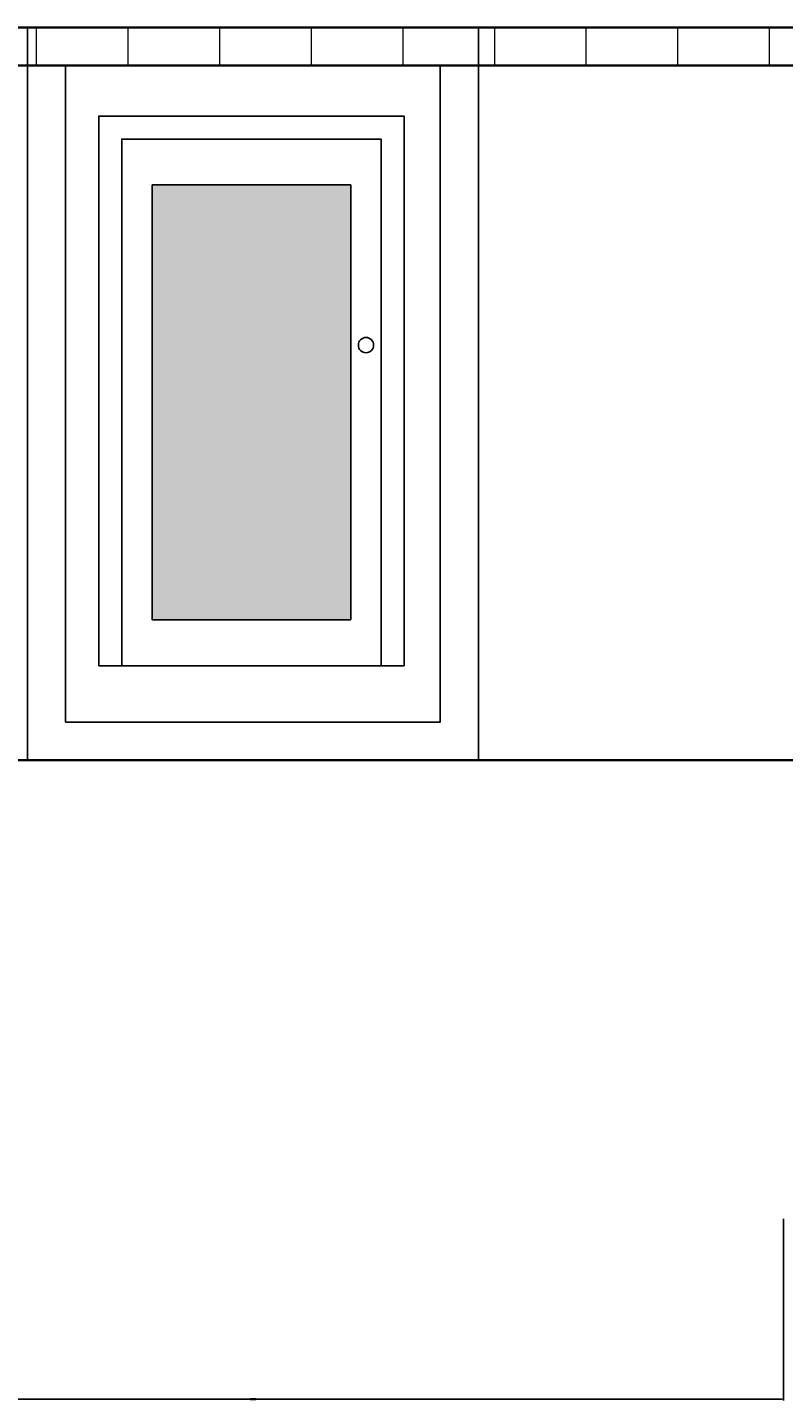
# Model space of a CAD drawing. Units: inches. Extents: x -128 to 854, y -395 to 398.
# Tile 11 of 61: x 23 to 122, y -382 to -202. Entities that reach past the tile are written whole.
import ezdxf

# ---------------------------------------------------------------- set-up
doc = ezdxf.new("R2010")
doc.units = ezdxf.units.IN
doc.header["$MEASUREMENT"] = 0
for name, color, linetype, lineweight in [('A-ANNO-DIMS', 2, 'Continuous', 18), ('A-DOOR', 4, 'Continuous', 25), ('A-SECT', 220, 'Continuous', 35), ('A-SECT-PATT', 8, 'Continuous', 13)]:
    doc.layers.add(name, color=color, linetype=linetype, lineweight=lineweight)
doc.styles.get("Standard").update_dxf_attribs({"font": 'arial.ttf'})
doc.dimstyles.get("Standard").update_dxf_attribs({"dimtxt": 0.18, "dimasz": 0.18, "dimexe": 0.18, "dimexo": 0.0625, "dimgap": 0.09, "dimtad": 0, "dimtih": 1, "dimtoh": 1, "dimdec": 1, "dimzin": 0, "dimdsep": 46, "dimlunit": 4, "dimtxsty": 'Standard', "dimcen": 0.09, "dimclrd": 1, "dimclre": 2, "dimclrt": 6, "dimadec": 0, "dimazin": 0, "dimtfac": 1, "dimtdec": 1, "dimtofl": 0, "dimtmove": 0, "dimatfit": 3, "dimfxl": 1, "dimtfill": 2, "dimtfillclr": 3, "dimtolj": 1, "dimtzin": 0, "dimarcsym": 0})

# ---------------------------------------------------------------- blocks, each defined once
blk = doc.blocks.new('*U59')
blk.add_lwpolyline([(3.12, 0.01), (0.12, 0.01), (0.12, 72.01), (40.12, 72.01), (40.12, 0.01), (37.12, 0.01)])
for points in [[(37.12, 68.99), (37.12, 0.01), (3.12, 0.01), (3.12, 68.99)], [(33.12, 6.01), (33.12, 62.99), (7.12, 62.99), (7.12, 6.01)]]:
    blk.add_lwpolyline(points, close=True)
blk.add_circle((35.12, 42.01), 1)
blk = doc.blocks.new('*D123')
at = {"layer": 'A-ANNO-DIMS', "color": 2, "lineweight": -2, "transparency": 16777216}
for p, q in [((-17.16, -358.08), (-17.16, -381.9)), ((121.84, -358.08), (121.84, -381.9))]:
    blk.add_line(p, q, dxfattribs=at)
at = {"layer": 'A-ANNO-DIMS', "color": 1, "lineweight": -2, "transparency": 16777216}
for p, q in [((-16.98, -381.72), (51.95, -381.72)), ((121.66, -381.72), (52.73, -381.72))]:
    blk.add_line(p, q, dxfattribs=at)
at = {"layer": 'A-ANNO-DIMS', "color": 1, "transparency": 16777216}
for points in [[(-16.98, -381.69), (-16.98, -381.75), (-17.16, -381.72)], [(121.66, -381.69), (121.66, -381.75), (121.84, -381.72)]]:
    blk.add_solid(points, dxfattribs=at)
at = {"layer": 'Defpoints', "color": 0, "transparency": 16777216}
for p in [(-17.16, -358.02), (121.84, -358.02), (121.84, -381.72)]:
    blk.add_point(p, dxfattribs=at)
at = {"layer": 'A-ANNO-DIMS', "color": 6, "transparency": 16777216, "insert": (52.34, -381.72), "char_height": 0.18, "attachment_point": 5, "bg_fill": 1, "box_fill_scale": 1.25, "bg_fill_color": 3, "bg_fill_transparency": 0}
blk.add_mtext('\\A1;11\'-7"', dxfattribs=at)

msp = doc.modelspace()

# ---------------------------------------------------------------- hatches: boundary and pattern name
at = {"layer": 'A-SECT-PATT'}
h = msp.add_hatch(dxfattribs=at)
h.set_pattern_fill('ANSI31', color=256, scale=96, angle=45, style=0)
h.paths.add_polyline_path([(-38.36, -202.02), (300.04, -202.02), (300.04, -207.02), (-38.36, -207.02)])
h = msp.add_hatch(color=256, dxfattribs=at)
h.dxf.hatch_style = 1
h.paths.add_polyline_path([(39.15, -279.63), (65.15, -279.63), (65.15, -222.65), (39.15, -222.65)])

# ---------------------------------------------------------------- linework, layer by layer
at = {"layer": 'A-DOOR'}
for points in [[(22.81, -202.02), (81.87, -202.02), (81.87, -298.02), (22.81, -298.02)], [(27.81, -207.02), (76.87, -207.02), (76.87, -293.02), (27.81, -293.02)]]:
    msp.add_lwpolyline(points, close=True, dxfattribs=at)
at = {"layer": 'A-SECT'}
for p, q in [((-56.16, -202.02), (317.84, -202.02)), ((-56.16, -207.02), (317.84, -207.02)), ((-56.16, -298.02), (312.84, -298.02))]:
    msp.add_line(p, q, dxfattribs=at)

# ---------------------------------------------------------------- block references
at = {"layer": 'A-DOOR'}
msp.add_blockref('*U59', (32.03, -285.64), dxfattribs=at)

# ---------------------------------------------------------------- dimensions: what is measured, and where the dimension line sits
at = {"layer": 'A-ANNO-DIMS'}
dim = msp.add_linear_dim(base=(121.84, -381.72), p1=(-17.16, -358.02), p2=(121.84, -358.02), dimstyle='Standard', override={"dimdec": 1, "dimlfac": 1, "dimrnd": 0, "dimzin": 1, "dimdsep": 46, "dimlunit": 4, "dimfrac": 2}, dxfattribs=at)
dim.commit()
dim.dimension.update_dxf_attribs({"geometry": '*D123', "text_midpoint": (52.34, -381.72)})

doc.saveas('drawing.dxf')
